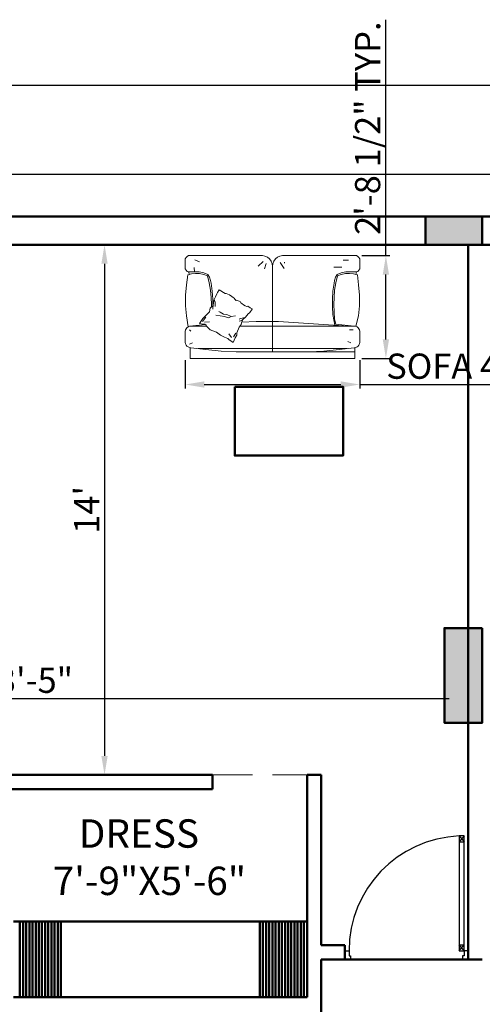
# Model space of a CAD drawing. Units: millimetres. Extents: x 1706 to 5913, y 156 to 1716.
# Tile 10 of 26: x 3377 to 3523, y 603 to 915. Entities that reach past the tile are written whole.
import ezdxf

# ---------------------------------------------------------------- set-up
doc = ezdxf.new("R2010")
doc.units = ezdxf.units.MM
doc.linetypes.add('DASHED', pattern=[19.05, 12.7, -6.35])
for name, color, linetype, lineweight in [('A-ANNO-DIMS', 2, 'Continuous', 18), ('A-AREA-IDEN', 3, 'Continuous', 18), ('A-COLS', 20, 'Continuous', 50), ('A-DOOR', 4, 'Continuous', 25), ('A-FLOR-OVHD', 9, 'DASHED', 18), ('A-FURN', 8, 'Continuous', 18), ('A-WALL', 7, 'Continuous', 50)]:
    doc.layers.add(name, color=color, linetype=linetype, lineweight=lineweight)
doc.styles.get("Standard").update_dxf_attribs({"font": 'arial.ttf'})
doc.dimstyles.new('ISO-25', dxfattribs={"dimtxt": 8, "dimasz": 6, "dimexe": 1.25, "dimexo": 0.625, "dimtad": 1, "dimdec": 0, "dimlunit": 3, "dimtxsty": 'Standard', "dimcen": 2.5, "dimadec": 0, "dimazin": 0, "dimtfac": 1, "dimtdec": 0, "dimtmove": 0, "dimatfit": 3, "dimfxl": 1, "dimarcsym": 0})

# ---------------------------------------------------------------- blocks, each defined once
blk = doc.blocks.new('Puerta 01')
for p, q in [((-0.7745, -0.0264), (-0.7368, -0.0584)), ((-0.7745, -0.0584), (-0.7368, -0.0264)), ((-0.7368, -0.0584), (-0.7368, -0.0264)), ((-0.028, -0.0584), (-0.0657, -0.0264)), ((-0.028, -0.0264), (-0.0657, -0.0584)), ((-0.0657, -0.0584), (-0.0657, -0.0264))]:
    blk.add_line(p, q)
for points in [[(-0.028, 0), (-0.028, -0.0264), (0.004, -0.0264), (0.004, -0.036), (0.028, -0.036), (0.028, 0)], [(-0.028, -0.0264), (-0.7745, -0.0264), (-0.7745, -0.0584), (-0.028, -0.0584)], [(0.004, -0.7736), (0.004, -0.764), (0.028, -0.764), (0.028, -0.8), (-0.028, -0.8), (-0.028, -0.7736)]]:
    blk.add_lwpolyline(points, close=True)
blk.add_arc((-0.028, -0.0264), 0.7472, 182.45453, 270)
blk = doc.blocks.new('sofa-44')
at = {"color": 0, "linetype": 'ByBlock'}
for p, q in [((-0.038, 0.929), (-0.045, 0.917)), ((-0.045, 0.917), (-0.038, 0.929)), ((-0.045, 0.917), (-0.045, 0.824)), ((-0.045, 0.917), (-0.045, 0.824)), ((-0.028, 0.939), (-0.038, 0.929)), ((-0.038, 0.929), (-0.028, 0.939)), ((-0.015, 0.947), (-0.028, 0.939)), ((-0.028, 0.939), (-0.015, 0.947)), ((-0.003, 0.947), (-0.015, 0.947)), ((-0.015, 0.947), (-0.003, 0.947)), ((0.665, 0.947), (-0.003, 0.947)), ((-0.003, 0.947), (0.665, 0.947)), ((0.042, 0.909), (0.087, 0.889)), ((0.687, 0.942), (0.665, 0.947)), ((0.687, 0.942), (0.665, 0.947)), ((0.712, 0.932), (0.687, 0.942)), ((0.712, 0.932), (0.687, 0.942)), ((0.73, 0.917), (0.712, 0.932)), ((0.73, 0.917), (0.712, 0.932)), ((0.745, 0.897), (0.73, 0.917)), ((0.745, 0.897), (0.73, 0.917)), ((0.785, 0.917), (0.77, 0.897)), ((0.77, 0.897), (0.785, 0.917)), ((0.805, 0.932), (0.785, 0.917)), ((0.785, 0.917), (0.805, 0.932)), ((0.827, 0.942), (0.805, 0.932)), ((0.805, 0.932), (0.827, 0.942)), ((0.85, 0.947), (0.827, 0.942)), ((0.827, 0.942), (0.85, 0.947)), ((1.52, 0.947), (0.85, 0.947)), ((0.85, 0.947), (1.52, 0.947)), ((1.532, 0.947), (1.52, 0.947)), ((1.532, 0.947), (1.52, 0.947)), ((1.545, 0.939), (1.532, 0.947)), ((1.545, 0.939), (1.532, 0.947)), ((1.555, 0.929), (1.545, 0.939)), ((1.555, 0.929), (1.545, 0.939)), ((1.562, 0.917), (1.555, 0.929)), ((1.562, 0.917), (1.555, 0.929)), ((1.562, 0.824), (1.562, 0.917)), ((1.562, 0.917), (1.562, 0.824)), ((-0.045, 0.824), (-0.038, 0.812)), ((-0.045, 0.824), (-0.038, 0.812)), ((0.04, 0.799), (0.037, 0.839)), ((0.672, 0.892), (0.627, 0.849)), ((0.7, 0.874), (0.685, 0.824)), ((0.755, 0.872), (0.745, 0.897)), ((0.755, 0.872), (0.745, 0.897)), ((0.757, 0.849), (0.755, 0.872)), ((0.757, 0.849), (0.755, 0.872)), ((0.76, 0.872), (0.757, 0.849)), ((0.757, 0.849), (0.76, 0.872)), ((0.757, 0.06), (0.757, 0.849)), ((0.77, 0.897), (0.76, 0.872)), ((0.76, 0.872), (0.77, 0.897)), ((0.83, 0.884), (0.867, 0.829)), ((0.87, 0.887), (0.87, 0.877)), ((1.397, 0.842), (1.322, 0.842)), ((1.46, 0.904), (1.41, 0.904)), ((1.555, 0.812), (1.562, 0.824)), ((1.562, 0.824), (1.555, 0.812)), ((-0.038, 0.812), (-0.028, 0.802)), ((-0.038, 0.812), (-0.028, 0.802)), ((-0.023, 0.769), (-0.035, 0.677)), ((-0.023, 0.769), (-0.035, 0.677)), ((-0.028, 0.802), (-0.015, 0.797)), ((-0.028, 0.802), (-0.015, 0.797)), ((0.012, 0.779), (-0.023, 0.769)), ((-0.0064, 0.7737), (-0.023, 0.769)), ((-0.015, 0.797), (-0.0064, 0.7737)), ((-0.015, 0.797), (-0.003, 0.797)), ((-0.0064, 0.7737), (-0.015, 0.797)), ((0.04, 0.799), (-0.003, 0.797)), ((0.05, 0.782), (0.012, 0.779)), ((0.082, 0.797), (0.04, 0.799)), ((0.087, 0.782), (0.05, 0.782)), ((0.125, 0.787), (0.082, 0.797)), ((0.125, 0.774), (0.087, 0.782)), ((0.162, 0.772), (0.125, 0.787)), ((0.16, 0.762), (0.125, 0.774)), ((0.175, 0.697), (0.16, 0.762)), ((0.177, 0.747), (0.162, 0.772)), ((0.187, 0.719), (0.177, 0.747)), ((1.33, 0.719), (1.34, 0.747)), ((1.34, 0.747), (1.355, 0.772)), ((1.342, 0.697), (1.357, 0.762)), ((1.355, 0.772), (1.392, 0.787)), ((1.357, 0.762), (1.392, 0.774)), ((1.392, 0.787), (1.435, 0.797)), ((1.392, 0.774), (1.43, 0.782)), ((1.43, 0.782), (1.467, 0.782)), ((1.435, 0.797), (1.477, 0.799)), ((1.467, 0.782), (1.505, 0.779)), ((1.477, 0.799), (1.52, 0.797)), ((1.505, 0.779), (1.54, 0.769)), ((1.532, 0.797), (1.52, 0.797)), ((1.5248, 0.7734), (1.532, 0.797)), ((1.5248, 0.7734), (1.532, 0.797)), ((1.54, 0.769), (1.5248, 0.7734)), ((1.532, 0.797), (1.545, 0.802)), ((1.545, 0.802), (1.532, 0.797)), ((1.552, 0.677), (1.54, 0.769)), ((1.54, 0.769), (1.552, 0.677)), ((1.545, 0.802), (1.555, 0.812)), ((1.555, 0.812), (1.545, 0.802)), ((-0.035, 0.677), (-0.043, 0.582)), ((-0.035, 0.677), (-0.043, 0.582)), ((0.187, 0.629), (0.175, 0.697)), ((0.192, 0.692), (0.187, 0.719)), ((0.202, 0.619), (0.192, 0.692)), ((1.315, 0.619), (1.325, 0.692)), ((1.325, 0.692), (1.33, 0.719)), ((1.33, 0.629), (1.342, 0.697)), ((1.56, 0.582), (1.552, 0.677)), ((1.552, 0.677), (1.56, 0.582)), ((-0.043, 0.582), (-0.043, 0.484)), ((-0.043, 0.582), (-0.043, 0.484)), ((0.192, 0.562), (0.187, 0.629)), ((0.195, 0.497), (0.192, 0.562)), ((0.207, 0.547), (0.202, 0.619)), ((0.207, 0.492), (0.207, 0.547)), ((0.232, 0.567), (0.222, 0.542)), ((0.245, 0.594), (0.232, 0.567)), ((0.252, 0.607), (0.245, 0.594)), ((0.267, 0.632), (0.252, 0.607)), ((0.322, 0.599), (0.267, 0.632)), ((0.332, 0.597), (0.322, 0.599)), ((0.362, 0.584), (0.332, 0.597)), ((0.385, 0.569), (0.362, 0.584)), ((0.397, 0.562), (0.385, 0.569)), ((0.405, 0.554), (0.397, 0.562)), ((0.42, 0.534), (0.405, 0.554)), ((1.31, 0.547), (1.315, 0.619)), ((1.31, 0.474), (1.31, 0.547)), ((1.322, 0.497), (1.325, 0.562)), ((1.325, 0.562), (1.33, 0.629)), ((1.56, 0.484), (1.56, 0.582)), ((1.56, 0.582), (1.56, 0.484)), ((-0.043, 0.484), (-0.035, 0.392)), ((-0.043, 0.484), (-0.035, 0.392)), ((0.185, 0.462), (0.177, 0.43)), ((0.192, 0.472), (0.185, 0.462)), ((0.212, 0.487), (0.192, 0.472)), ((0.195, 0.482), (0.195, 0.497)), ((0.207, 0.467), (0.212, 0.487)), ((0.207, 0.452), (0.207, 0.467)), ((0.215, 0.514), (0.212, 0.487)), ((0.222, 0.542), (0.215, 0.514)), ((0.222, 0.542), (0.23, 0.519)), ((0.23, 0.519), (0.23, 0.497)), ((0.23, 0.497), (0.23, 0.477)), ((0.425, 0.537), (0.42, 0.534)), ((0.46, 0.524), (0.425, 0.537)), ((0.467, 0.512), (0.46, 0.524)), ((0.475, 0.507), (0.467, 0.512)), ((0.492, 0.492), (0.475, 0.507)), ((0.507, 0.484), (0.492, 0.492)), ((0.522, 0.479), (0.507, 0.484)), ((0.532, 0.482), (0.522, 0.479)), ((0.552, 0.467), (0.532, 0.482)), ((0.57, 0.457), (0.552, 0.467)), ((0.572, 0.452), (0.57, 0.457)), ((1.315, 0.405), (1.31, 0.474)), ((1.325, 0.43), (1.322, 0.497)), ((1.552, 0.392), (1.56, 0.484)), ((1.56, 0.484), (1.552, 0.392)), ((-0.035, 0.392), (-0.02, 0.292)), ((-0.035, 0.392), (-0.02, 0.292)), ((0.117, 0.367), (0.087, 0.322)), ((0.112, 0.34), (0.145, 0.38)), ((0.145, 0.395), (0.117, 0.367)), ((0.177, 0.43), (0.145, 0.395)), ((0.237, 0.397), (0.315, 0.385)), ((0.277, 0.425), (0.265, 0.432)), ((0.307, 0.407), (0.277, 0.425)), ((0.337, 0.405), (0.307, 0.407)), ((0.315, 0.385), (0.352, 0.375)), ((0.377, 0.387), (0.337, 0.405)), ((0.352, 0.375), (0.377, 0.387)), ((0.377, 0.387), (0.417, 0.392)), ((0.462, 0.367), (0.452, 0.36)), ((0.505, 0.377), (0.462, 0.367)), ((0.485, 0.357), (0.505, 0.377)), ((0.505, 0.377), (0.525, 0.397)), ((0.525, 0.397), (0.532, 0.407)), ((0.532, 0.407), (0.55, 0.422)), ((0.55, 0.422), (0.572, 0.452)), ((1.3327, 0.3055), (1.315, 0.405)), ((1.33, 0.362), (1.325, 0.43)), ((1.525, 0.297), (1.552, 0.392)), ((1.552, 0.392), (1.525, 0.297)), ((-0.03, 0.282), (-0.038, 0.272)), ((-0.03, 0.282), (-0.038, 0.272)), ((-0.02, 0.292), (-0.03, 0.282)), ((-0.02, 0.292), (-0.03, 0.282)), ((-0.008, 0.297), (-0.02, 0.292)), ((0.14, 0.312), (-0.008, 0.297)), ((-0.008, 0.297), (0.15, 0.297)), ((0.005, 0.297), (-0.008, 0.297)), ((0.087, 0.322), (0.1, 0.317)), ((0.1, 0.317), (0.135, 0.315)), ((0.132, 0.335), (0.177, 0.337)), ((0.135, 0.315), (0.147, 0.307)), ((0.147, 0.307), (0.152, 0.295)), ((0.152, 0.295), (0.185, 0.262)), ((0.43, 0.235), (0.452, 0.287)), ((0.477, 0.35), (0.452, 0.342)), ((0.452, 0.287), (0.47, 0.312)), ((0.46, 0.297), (1.525, 0.297)), ((0.467, 0.307), (0.462, 0.307)), ((0.47, 0.312), (0.472, 0.327)), ((0.472, 0.327), (0.485, 0.357)), ((0.607, 0.34), (0.475, 0.335)), ((0.485, 0.357), (0.477, 0.35)), ((0.815, 0.34), (0.607, 0.34)), ((1.46, 0.297), (0.815, 0.34)), ((1.3414, 0.3143), (1.33, 0.362)), ((1.512, 0.297), (1.3414, 0.3143)), ((1.537, 0.292), (1.525, 0.297)), ((1.537, 0.292), (1.525, 0.297)), ((1.547, 0.282), (1.537, 0.292)), ((1.547, 0.282), (1.537, 0.292)), ((1.555, 0.272), (1.547, 0.282)), ((1.555, 0.272), (1.547, 0.282)), ((-0.043, 0.262), (-0.045, 0.247)), ((-0.043, 0.262), (-0.045, 0.247)), ((-0.045, 0.247), (-0.045, 0.147)), ((-0.045, 0.247), (-0.045, 0.147)), ((-0.038, 0.272), (-0.043, 0.262)), ((-0.038, 0.272), (-0.043, 0.262)), ((-0.005, 0.262), (0.007, 0.25)), ((0.185, 0.262), (0.242, 0.242)), ((0.242, 0.242), (0.28, 0.215)), ((0.28, 0.215), (0.317, 0.195)), ((0.317, 0.195), (0.347, 0.182)), ((0.347, 0.182), (0.357, 0.175)), ((0.38, 0.192), (0.355, 0.225)), ((0.397, 0.147), (0.415, 0.19)), ((0.4, 0.197), (0.42, 0.232)), ((0.415, 0.19), (0.43, 0.215)), ((0.43, 0.215), (0.43, 0.235)), ((1.502, 0.262), (1.467, 0.262)), ((1.56, 0.262), (1.555, 0.272)), ((1.56, 0.262), (1.555, 0.272)), ((1.562, 0.247), (1.56, 0.262)), ((1.562, 0.247), (1.56, 0.262)), ((1.562, 0.147), (1.562, 0.247)), ((1.562, 0.147), (1.562, 0.247)), ((-0.045, 0.147), (-0.043, 0.135)), ((-0.045, 0.147), (-0.043, 0.135)), ((-0.043, 0.135), (-0.038, 0.122)), ((-0.043, 0.135), (-0.038, 0.122)), ((-0.038, 0.122), (-0.03, 0.112)), ((-0.038, 0.122), (-0.03, 0.112)), ((-0.03, 0.112), (-0.02, 0.105)), ((-0.03, 0.112), (-0.02, 0.105)), ((-0.02, 0.105), (-0.008, 0.1)), ((-0.02, 0.105), (-0.008, 0.1)), ((-0.008, 0.132), (0.02, 0.142)), ((-0.008, 0.1), (0, 0.0982)), ((-0.008, 0.1), (0.005, 0.097)), ((0, 0.1), (0, 0)), ((0, 0.0982), (0, 0)), ((0.005, 0.097), (0.145, 0.08)), ((0.357, 0.175), (0.397, 0.147)), ((1.372, 0.08), (1.512, 0.097)), ((1.48, 0.142), (1.452, 0.155)), ((1.512, 0.097), (1.525, 0.1)), ((1.517, 0.0982), (1.525, 0.1)), ((1.517, 0.1), (1.517, 0)), ((1.517, 0), (1.517, 0.0982)), ((1.525, 0.1), (1.537, 0.105)), ((1.525, 0.1), (1.537, 0.105)), ((1.537, 0.105), (1.547, 0.112)), ((1.537, 0.105), (1.547, 0.112)), ((1.547, 0.112), (1.555, 0.122)), ((1.547, 0.112), (1.555, 0.122)), ((1.555, 0.122), (1.56, 0.135)), ((1.555, 0.122), (1.56, 0.135)), ((1.56, 0.135), (1.562, 0.147)), ((1.56, 0.135), (1.562, 0.147)), ((0, 0), (1.517, 0)), ((0, 0), (1.517, 0)), ((0.072, 0.09), (0.752, 0.09)), ((0.145, 0.08), (0.285, 0.067)), ((0.285, 0.067), (0.425, 0.06)), ((0.425, 0.06), (1.517, 0.06)), ((0.752, 0.09), (0.765, 0.09)), ((0.765, 0.09), (1.445, 0.09)), ((1.092, 0.06), (1.232, 0.067)), ((1.232, 0.067), (1.372, 0.08))]:
    blk.add_line(p, q, dxfattribs=at)
blk = doc.blocks.new('*D151')
at = {"layer": 'A-ANNO-DIMS', "color": 0, "lineweight": -2, "transparency": 16777216}
for p, q in [((3405.67, 843.39), (3402.28, 843.39)), ((3403.53, 837.39), (3403.53, 681.39)), ((3405.67, 675.39), (3402.28, 675.39))]:
    blk.add_line(p, q, dxfattribs=at)
at = {"layer": 'A-ANNO-DIMS', "color": 0, "transparency": 16777216}
for points in [[(3402.53, 837.39), (3404.53, 837.39), (3403.53, 843.39)], [(3402.53, 681.39), (3404.53, 681.39), (3403.53, 675.39)]]:
    blk.add_solid(points, dxfattribs=at)
at = {"layer": 'Defpoints', "color": 0, "transparency": 16777216}
for p in [(3406.3, 843.39), (3403.53, 675.39), (3406.3, 675.39)]:
    blk.add_point(p, dxfattribs=at)
at = {"layer": 'A-ANNO-DIMS', "color": 0, "transparency": 16777216, "insert": (3398.89, 759.39), "char_height": 8, "attachment_point": 5, "rotation": 90}
blk.add_mtext("14'", dxfattribs=at)
blk = doc.blocks.new('*D152')
at = {"layer": 'A-ANNO-DIMS', "color": 0, "lineweight": -2, "transparency": 16777216}
for p, q in [((3238.21, 715.75), (3238.21, 698.36)), ((3518.71, 715.75), (3518.71, 698.36)), ((3244.21, 699.61), (3512.71, 699.61))]:
    blk.add_line(p, q, dxfattribs=at)
at = {"layer": 'A-ANNO-DIMS', "color": 0, "transparency": 16777216}
for points in [[(3244.21, 700.61), (3244.21, 698.61), (3238.21, 699.61)], [(3512.71, 700.61), (3512.71, 698.61), (3518.71, 699.61)]]:
    blk.add_solid(points, dxfattribs=at)
at = {"layer": 'Defpoints', "color": 0, "transparency": 16777216}
for p in [(3238.21, 716.38), (3518.71, 716.38), (3518.71, 699.61)]:
    blk.add_point(p, dxfattribs=at)
at = {"layer": 'A-ANNO-DIMS', "color": 0, "transparency": 16777216, "insert": (3378.46, 704.33), "char_height": 8, "attachment_point": 5}
blk.add_mtext('23\'-5"', dxfattribs=at)
blk = doc.blocks.new('*D146')
at = {"layer": 'A-ANNO-DIMS', "color": 0, "lineweight": -2, "transparency": 16777216}
for p, q in [((3238.21, 853.01), (3238.21, 866.93)), ((3934.32, 865.68), (3244.21, 865.68)), ((3940.32, 853.01), (3940.32, 866.93))]:
    blk.add_line(p, q, dxfattribs=at)
at = {"layer": 'A-ANNO-DIMS', "color": 0, "transparency": 16777216}
for points in [[(3244.21, 866.68), (3244.21, 864.68), (3238.21, 865.68)], [(3934.32, 866.68), (3934.32, 864.68), (3940.32, 865.68)]]:
    blk.add_solid(points, dxfattribs=at)
at = {"layer": 'Defpoints', "color": 0, "transparency": 16777216}
for p in [(3238.21, 865.68), (3238.21, 852.39), (3940.32, 852.39)]:
    blk.add_point(p, dxfattribs=at)
at = {"layer": 'A-ANNO-DIMS', "color": 0, "transparency": 16777216, "insert": (3589.27, 870.39), "char_height": 8, "attachment_point": 5}
blk.add_mtext('58\'-6"', dxfattribs=at)
blk = doc.blocks.new('*D148')
at = {"layer": 'A-ANNO-DIMS', "color": 0, "lineweight": -2, "transparency": 16777216}
for p, q in [((3184.21, 853.01), (3184.21, 895.24)), ((3190.21, 893.99), (4073.51, 893.99)), ((4079.51, 853.01), (4079.51, 895.24))]:
    blk.add_line(p, q, dxfattribs=at)
at = {"layer": 'A-ANNO-DIMS', "color": 0, "transparency": 16777216}
for points in [[(3190.21, 894.99), (3190.21, 892.99), (3184.21, 893.99)], [(4073.51, 894.99), (4073.51, 892.99), (4079.51, 893.99)]]:
    blk.add_solid(points, dxfattribs=at)
at = {"layer": 'Defpoints', "color": 0, "transparency": 16777216}
for p in [(4079.51, 893.99), (3184.21, 852.39), (4079.51, 852.39)]:
    blk.add_point(p, dxfattribs=at)
at = {"layer": 'A-ANNO-DIMS', "color": 0, "transparency": 16777216, "insert": (3631.86, 898.61), "char_height": 8, "attachment_point": 5}
blk.add_mtext('74\'-7"', dxfattribs=at)
blk = doc.blocks.new('*D223')
at = {"layer": 'A-ANNO-DIMS', "color": 0, "lineweight": -2, "transparency": 16777216}
for p, q in [((3429.12, 806.8), (3429.12, 797.88)), ((3484.38, 806.8), (3484.38, 797.88)), ((3435.12, 799.13), (3478.38, 799.13)), ((3484.38, 799.13), (3592.53, 799.13))]:
    blk.add_line(p, q, dxfattribs=at)
at = {"layer": 'A-ANNO-DIMS', "color": 0, "transparency": 16777216}
for points in [[(3435.12, 800.13), (3435.12, 798.13), (3429.12, 799.13)], [(3478.38, 800.13), (3478.38, 798.13), (3484.38, 799.13)]]:
    blk.add_solid(points, dxfattribs=at)
at = {"layer": 'Defpoints', "color": 0, "transparency": 16777216}
for p in [(3429.12, 807.42), (3484.38, 807.42), (3484.38, 799.13)]:
    blk.add_point(p, dxfattribs=at)
at = {"layer": 'A-ANNO-DIMS', "color": 0, "transparency": 16777216, "insert": (3541.46, 803.9), "char_height": 8, "attachment_point": 5}
blk.add_mtext('SOFA 4\'-7 1/2" TYP.', dxfattribs=at)
blk = doc.blocks.new('*D224')
at = {"layer": 'A-ANNO-DIMS', "color": 0, "lineweight": -2, "transparency": 16777216}
for p, q in [((3492.67, 839.99), (3492.67, 914.78)), ((3485.01, 839.99), (3493.92, 839.99)), ((3492.67, 813.42), (3492.67, 833.99)), ((3485.01, 807.42), (3493.92, 807.42))]:
    blk.add_line(p, q, dxfattribs=at)
at = {"layer": 'A-ANNO-DIMS', "color": 0, "transparency": 16777216}
for points in [[(3491.67, 833.99), (3493.67, 833.99), (3492.67, 839.99)], [(3491.67, 813.42), (3493.67, 813.42), (3492.67, 807.42)]]:
    blk.add_solid(points, dxfattribs=at)
at = {"layer": 'Defpoints', "color": 0, "transparency": 16777216}
for p in [(3484.38, 839.99), (3492.67, 839.99), (3484.38, 807.42)]:
    blk.add_point(p, dxfattribs=at)
at = {"layer": 'A-ANNO-DIMS', "color": 0, "transparency": 16777216, "insert": (3487.91, 880.38), "char_height": 8, "attachment_point": 5, "rotation": 90}
blk.add_mtext('2\'-8 1/2" TYP.', dxfattribs=at)

msp = doc.modelspace()

# ---------------------------------------------------------------- hatches: boundary and pattern name
at = {"layer": 'A-COLS'}
h = msp.add_hatch(color=256, dxfattribs=at)
h.dxf.hatch_style = 1
h.paths.add_polyline_path([(3523.21, 852.39), (3505.21, 852.39), (3505.21, 843.39), (3523.21, 843.39)])
h = msp.add_hatch(color=256, dxfattribs=at)
h.dxf.hatch_style = 1
h.paths.add_polyline_path([(3523.21, 721.89), (3511.21, 721.89), (3511.21, 691.89), (3523.21, 691.89)])

# ---------------------------------------------------------------- linework, layer by layer
for points in [[(3523.21, 852.39), (3505.21, 852.39), (3505.21, 843.39), (3523.21, 843.39)], [(3523.21, 721.89), (3511.21, 721.89), (3511.21, 691.89), (3523.21, 691.89)]]:
    msp.add_lwpolyline(points, close=True, dxfattribs=at)
at = {"layer": 'A-FLOR-OVHD'}
msp.add_line((3437.71, 675.39), (3467.71, 675.39), dxfattribs=at)
at = {"layer": 'A-WALL'}
for p, q in [((3209.71, 852.39), (4024.21, 852.39)), ((3505.21, 843.39), (3505.21, 852.39)), ((3214.21, 843.39), (3611.71, 843.39)), ((3518.71, 843.39), (3518.71, 616.89)), ((3511.21, 691.89), (3511.21, 721.89)), ((3511.21, 721.89), (3523.21, 721.89)), ((3238.21, 675.39), (3437.71, 675.39)), ((3437.71, 675.39), (3437.71, 670.89)), ((3467.71, 675.39), (3467.71, 604.89)), ((3467.71, 675.39), (3472.21, 675.39)), ((3472.21, 675.39), (3472.21, 621.39)), ((3238.21, 670.89), (3437.71, 670.89)), ((3374.71, 628.89), (3467.71, 628.89)), ((3376.71, 628.89), (3376.71, 604.89)), ((3377.71, 628.89), (3377.71, 604.89)), ((3378.71, 628.89), (3378.71, 604.89)), ((3379.71, 628.89), (3379.71, 604.89)), ((3380.71, 628.89), (3380.71, 604.89)), ((3381.71, 628.89), (3381.71, 604.89)), ((3382.71, 628.89), (3382.71, 604.89)), ((3383.71, 628.89), (3383.71, 604.89)), ((3384.71, 628.89), (3384.71, 604.89)), ((3385.71, 628.89), (3385.71, 604.89)), ((3386.71, 628.89), (3386.71, 604.89)), ((3387.71, 628.89), (3387.71, 604.89)), ((3388.71, 628.89), (3388.71, 604.89)), ((3389.71, 628.89), (3389.71, 604.89)), ((3452.71, 628.89), (3452.71, 604.89)), ((3453.71, 628.89), (3453.71, 604.89)), ((3454.71, 628.89), (3454.71, 604.89)), ((3455.71, 628.89), (3455.71, 604.89)), ((3456.71, 628.89), (3456.71, 604.89)), ((3457.71, 628.89), (3457.71, 604.89)), ((3458.71, 628.89), (3458.71, 604.89)), ((3459.71, 628.89), (3459.71, 604.89)), ((3460.71, 628.89), (3460.71, 604.89)), ((3461.71, 628.89), (3461.71, 604.89)), ((3462.71, 628.89), (3462.71, 604.89)), ((3463.71, 628.89), (3463.71, 604.89)), ((3464.71, 628.89), (3464.71, 604.89)), ((3465.71, 628.89), (3465.71, 604.89)), ((3466.71, 628.89), (3466.71, 604.89)), ((3472.21, 621.39), (3479.71, 621.39)), ((3479.71, 621.39), (3479.71, 616.89)), ((3472.21, 616.89), (3472.21, 556.89)), ((3472.21, 616.89), (3479.71, 616.89)), ((3479.71, 616.89), (3518.71, 616.89)), ((3518.71, 616.89), (3523.21, 616.89)), ((3374.71, 604.89), (3467.71, 604.89))]:
    msp.add_line(p, q, dxfattribs=at)
msp.add_lwpolyline([(3444.78, 798.43), (3479.12, 798.43), (3479.12, 776.6), (3444.78, 776.6)], close=True, dxfattribs=at)

# ---------------------------------------------------------------- block references
at = {"layer": 'A-DOOR', "xscale": 48.75000000000289, "yscale": 48.75000000000289, "zscale": 48.75000000000289, "rotation": 270.0000000012045}
msp.add_blockref('Puerta 01', (3518.71, 618.25), dxfattribs=at)
at = {"layer": 'A-FURN', "xscale": 34.38766350546327, "yscale": 34.38766350546327, "zscale": 34.38766350546327}
msp.add_blockref('sofa-44', (3430.67, 807.42), dxfattribs=at)

# ---------------------------------------------------------------- texts
at = {"layer": 'A-AREA-IDEN', "insert": (3381.61, 661.28), "char_height": 9, "attachment_point": 1}
msp.add_mtext_dynamic_manual_height_columns('     DRESS\\P  7\'-9"X5\'-6"', width=67.9131, gutter_width=12.5, heights=[0], dxfattribs=at)

# ---------------------------------------------------------------- dimensions: what is measured, and where the dimension line sits
at = {"layer": 'A-ANNO-DIMS'}
dim = msp.add_linear_dim(base=(3492.67, 839.99), p1=(3484.38, 807.42), p2=(3484.38, 839.99), angle=90, text='<> TYP.', dimstyle='ISO-25', override={"dimdec": 1, "dimrnd": 0, "dimzin": 1, "dimlunit": 4, "dimfrac": 2}, dxfattribs=at)
dim.commit()
dim.dimension.update_dxf_attribs({"geometry": '*D224', "text_midpoint": (3487.91, 880.38)})
for base, p1, p2, picture, middle in [((4079.51, 893.99), (3184.21, 852.39), (4079.51, 852.39), '*D148', (3631.86, 898.61)), ((3238.21, 865.68), (3940.32, 852.39), (3238.21, 852.39), '*D146', (3589.27, 870.39)), ((3518.71347462, 699.61377739), (3238.21347462, 716.37940041), (3518.71347462, 716.37940041), '*D152', (3378.46347462, 704.32608981))]:
    dim = msp.add_linear_dim(base=base, p1=p1, p2=p2, dimstyle='ISO-25', override={"dimclrd": 0, "dimclre": 0, "dimclrt": 0}, dxfattribs=at)
    dim.commit()
    dim.dimension.update_dxf_attribs({"geometry": picture, "text_midpoint": middle})
dim = msp.add_linear_dim(base=(3403.53, 675.39), p1=(3406.3, 843.39), p2=(3406.3, 675.39), angle=90, dimstyle='ISO-25', override={"dimclrd": 0, "dimclre": 0, "dimclrt": 0}, dxfattribs=at)
dim.commit()
dim.dimension.update_dxf_attribs({"geometry": '*D151', "text_midpoint": (3398.89, 759.39)})
dim = msp.add_linear_dim(base=(3484.38, 799.13), p1=(3429.12, 807.42), p2=(3484.38, 807.42), text='SOFA <> TYP.', dimstyle='ISO-25', override={"dimdec": 1, "dimrnd": 0, "dimzin": 1, "dimlunit": 4, "dimfrac": 2}, dxfattribs=at)
dim.commit()
dim.dimension.update_dxf_attribs({"geometry": '*D223', "text_midpoint": (3541.46, 803.9)})

doc.saveas('drawing.dxf')
